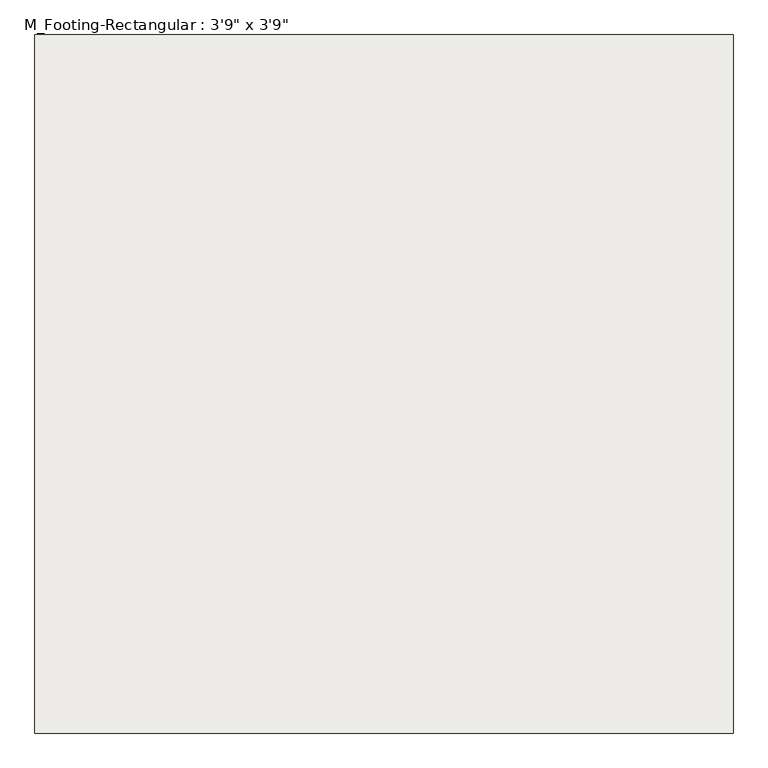
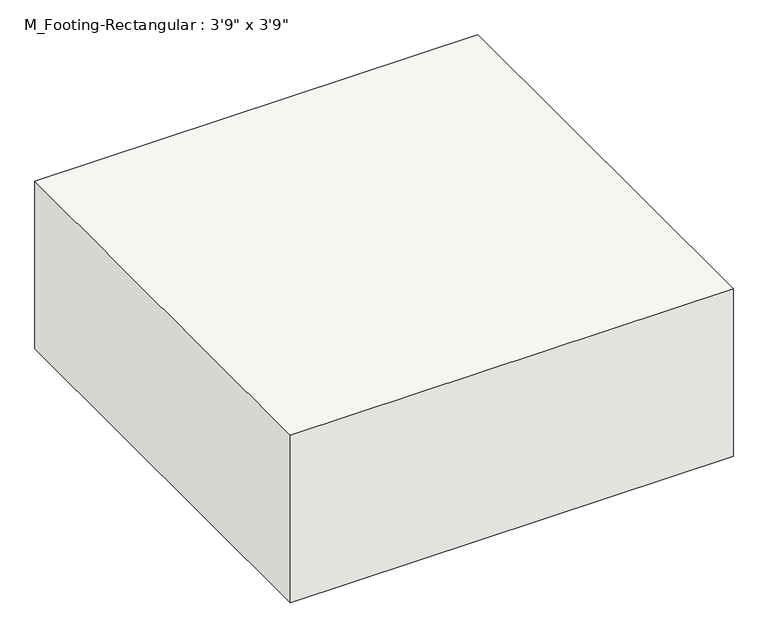
"""IFC4 building model written with IfcOpenShell, lengths in millimetres: slab geometry."""

from ifc_helpers import new_model, si_unit, frame, origin, place, context, project, spatial, polyline, outline, extrude, source, transform, mapped, element, save


def slab_90c2f4b8(model_context):
    return source(origin(), model_context, "Body", "SweptSolid", [
        extrude(outline(polyline([(571.5, 571.5), (571.5, -571.5), (-571.5, -571.5), (-571.5, 571.5), (571.5, 571.5)])), frame((0.0, 0.0, -457.2), z_axis=(0.0, 0.0, 1.0), x_axis=(1.0, 0.0, 0.0)), (0.0, 0.0, 1.0), 457.2),
    ])


if __name__ == "__main__":
    model = new_model("IFC4")
    model_context = context("Model", 3, world=origin())
    ifc_project = project(units=[si_unit("LENGTHUNIT", "METRE", prefix="MILLI")], contexts=[model_context])
    site = spatial("IfcSite", under=ifc_project)
    building = spatial("IfcBuilding", under=site)
    placement = place(None, origin())
    slab_shape = slab_90c2f4b8(model_context)
    element("IfcSlab", 1, ObjectType="M_Footing-Rectangular : 3'9\" x 3'9\"", at=placement, inside=building, context=model_context, shape_type="MappedRepresentation", body=[
        mapped(slab_shape, transform((0.0, 0.0, 0.0), x_axis=(1.0, 0.0, 0.0), y_axis=(0.0, 1.0, 0.0), z_axis=(0.0, 0.0, 1.0))),
    ])
    save(model, "model.ifc")

# Revit data of these elements
# Type "M_Footing-Rectangular : 3'9\" x 3'9\""
#   Width = 1143 mm
#   Length = 1143 mm
#   Foundation Thickness = 457.2 mm
#   Structural Material [instance default] = Concrete, Cast-in-Place gray
#   Assembly Code = ""
# Element 1 (IfcSlab, "M_Footing-Rectangular : 3'9\" x 3'9\"")
#   Materials on its faces: "Concrete, Cast-in-Place gray"
# Materials
#   "Concrete, Cast-in-Place gray": class "Concrete", colour RGB 192 192 192, transparency 0, Description = "Cast-in-place concrete", Cost = 0
